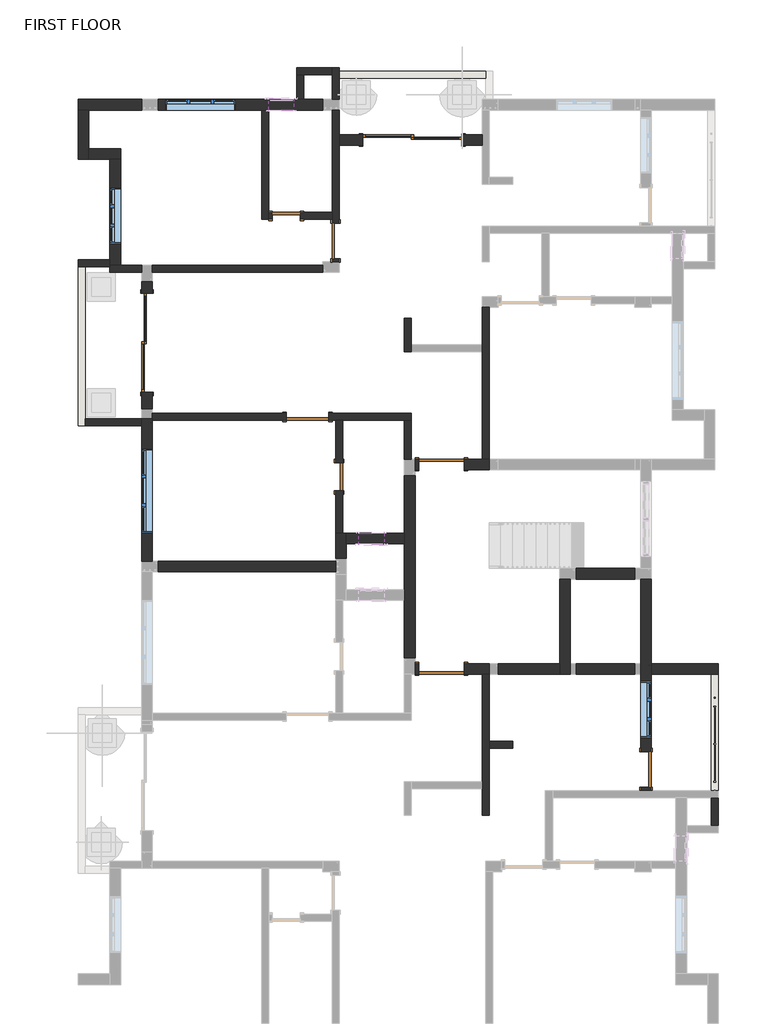
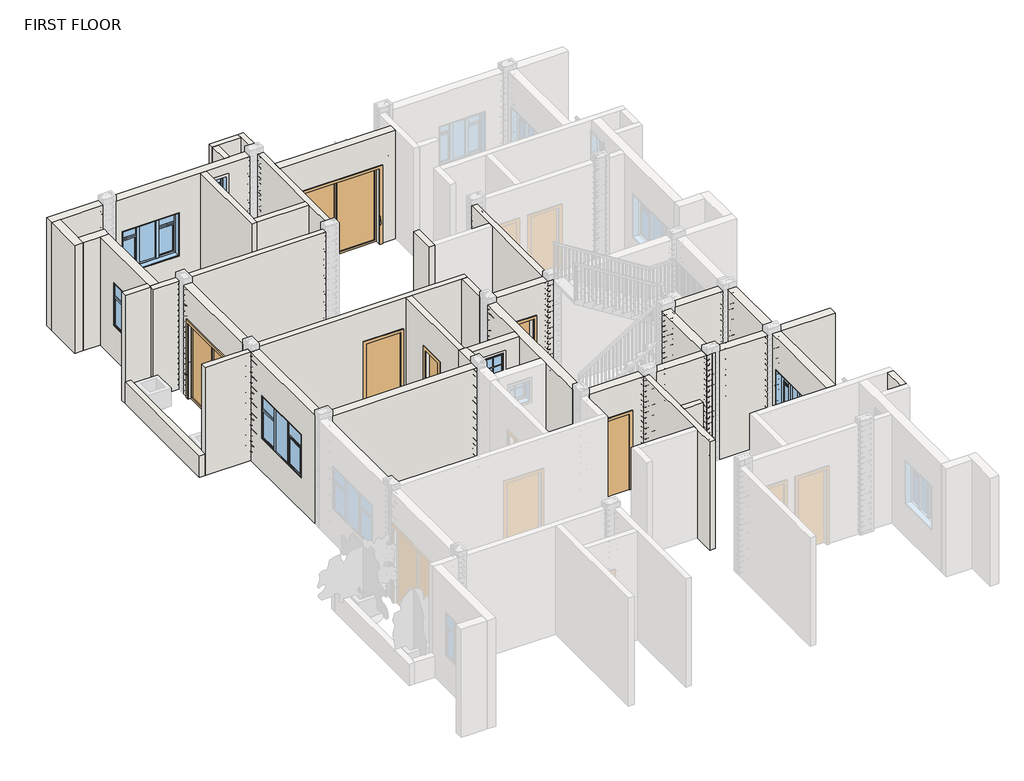
# One storey, part 2 of 10: 41 walls, 9 doors, 6 windows.
"""IFC4 building model written with IfcOpenShell, lengths in millimetres."""

from ifc_helpers import new_model, si_unit, frame, origin, place, context, project, spatial, polyline, outline, extrude, faceted_brep, transform, mapped, element, save
from components import door_double_sliding_7_x7_ddbaaa7c, door_e2b13fe9, door_bb98abfd, single_flush_2_x7_5ca4d175, door_ddcbdd8b, door_49933fe7, single_flush_3_x7_686f89d2, window_casement_triple_side_transom_4_x4_2_fd24aed3, window_casement_triple_side_transom_5_x4_f59ddf0b, window_casement_triple_side_transom_6_x4_596ba82f, window_6ec6991e

model = new_model("IFC4")

# Units and contexts
model_context = context("Model", 3, world=origin())
ifc_project = project(units=[si_unit("LENGTHUNIT", "METRE", prefix="MILLI")], contexts=[model_context])

# Site, building, storey
site = spatial("IfcSite", under=ifc_project)
building = spatial("IfcBuilding", under=site)
storey = spatial("IfcBuildingStorey", under=building, Name="FIRST FLOOR", Elevation=3200.4)

# Doors
placement = place(None, origin())
door_double_sliding_7_x7_shape = door_double_sliding_7_x7_ddbaaa7c(model_context)
element("IfcDoor", 1, ObjectType="Door-Double-Sliding : 7'X7'", at=placement, inside=storey, context=model_context, shape_type="MappedRepresentation", body=[
    mapped(door_double_sliding_7_x7_shape, transform((-403.8333787, 9140.759934, 3200.4), x_axis=(1.0, 0.0, 0.0), y_axis=(0.0, 1.0, 0.0), z_axis=(0.0, 0.0, 1.0))),
])
element("IfcDoor", 2, ObjectType="Door-Double-Sliding : 7'X7'", at=placement, inside=storey, context=model_context, shape_type="MappedRepresentation", body=[
    mapped(door_double_sliding_7_x7_shape, transform((-6010.8833787, 4886.259934, 3200.4), x_axis=(0.0, 1.0, 0.0), y_axis=(-1.0, 0.0, 0.0), z_axis=(0.0, 0.0, 1.0))),
])
door_shape = door_e2b13fe9(model_context)
element("IfcDoor", 3, ObjectType="Single-Flush : 2'6\"X7'", at=placement, inside=storey, context=model_context, shape_type="MappedRepresentation", body=[
    mapped(door_shape, transform((-2061.1833787, 7083.359934, 3200.4), x_axis=(0.0, -1.0, 0.0), y_axis=(1.0, 0.0, 0.0), z_axis=(0.0, 0.0, 1.0))),
])
door_2_shape = door_bb98abfd(model_context)
element("IfcDoor", 4, ObjectType="Single-Flush : 2'6\"X7'", at=placement, inside=storey, context=model_context, shape_type="MappedRepresentation", body=[
    mapped(door_2_shape, transform((4644.4166213, -4333.940066, 3200.4), x_axis=(0.0, -1.0, 0.0), y_axis=(1.0, 0.0, 0.0), z_axis=(0.0, 0.0, 1.0))),
])
single_flush_2_x7_shape = single_flush_2_x7_5ca4d175(model_context)
element("IfcDoor", 5, ObjectType="Single-Flush : 2'X7'", at=placement, inside=storey, context=model_context, shape_type="MappedRepresentation", body=[
    mapped(single_flush_2_x7_shape, transform((-3127.9833787, 7629.459934, 3200.4), x_axis=(-1.0, 0.0, 0.0), y_axis=(0.0, -1.0, 0.0), z_axis=(0.0, 0.0, 1.0))),
])
element("IfcDoor", 6, ObjectType="Single-Flush : 2'X7'", at=placement, inside=storey, context=model_context, shape_type="MappedRepresentation", body=[
    mapped(single_flush_2_x7_shape, transform((-1984.9833787, 1990.659934, 3200.4), x_axis=(0.0, 1.0, 0.0), y_axis=(-1.0, 0.0, 0.0), z_axis=(0.0, 0.0, 1.0))),
])
door_3_shape = door_ddcbdd8b(model_context)
element("IfcDoor", 7, ObjectType="Single-Flush : 3'3\"X7'", at=placement, inside=storey, context=model_context, shape_type="MappedRepresentation", body=[
    mapped(door_3_shape, transform((224.8166213, -2162.240066, 3200.4), x_axis=(-1.0, 0.0, 0.0), y_axis=(0.0, -1.0, 0.0), z_axis=(0.0, 0.0, 1.0))),
])
door_4_shape = door_49933fe7(model_context)
element("IfcDoor", 8, ObjectType="Single-Flush : 3'3\"X7'", at=placement, inside=storey, context=model_context, shape_type="MappedRepresentation", body=[
    mapped(door_4_shape, transform((224.8166213, 2257.359934, 3200.4), x_axis=(-1.0, 0.0, 0.0), y_axis=(0.0, -1.0, 0.0), z_axis=(0.0, 0.0, 1.0))),
])
single_flush_3_x7_shape = single_flush_3_x7_686f89d2(model_context)
element("IfcDoor", 9, ObjectType="Single-Flush : 3'X7'", at=placement, inside=storey, context=model_context, shape_type="MappedRepresentation", body=[
    mapped(single_flush_3_x7_shape, transform((-2670.7833787, 3286.059934, 3200.4), x_axis=(1.0, 0.0, 0.0), y_axis=(0.0, 1.0, 0.0), z_axis=(0.0, 0.0, 1.0))),
])

# Walls
element("IfcWall", 10, ObjectType="6\"", at=placement, inside=storey, context=model_context, shape_type="Brep", body=[
    faceted_brep([(-3661.3833787, 9915.459934, 3200.4), (-3661.3833787, 7553.259934, 3200.4), (-3661.3833787, 7553.259934, 6248.4), (-3661.3833787, 9915.459934, 6248.4), (-3508.9833787, 9915.459934, 3200.4), (-3508.9833787, 9915.459934, 5334.0), (-3508.9833787, 9915.459934, 5943.6), (-3508.9833787, 9915.459934, 6248.4), (-3508.9833787, 7705.659934, 6248.4), (-3508.9833787, 7553.259934, 6248.4), (-3508.9833787, 7553.259934, 3200.4), (-3508.9833787, 7705.659934, 3200.4)], [[[0, 1, 2, 3]], [[4, 5, 6, 7, 8, 9, 10, 11]], [[1, 0, 4, 11, 10]], [[3, 2, 9, 8, 7]], [[0, 3, 7, 6, 5, 4]], [[2, 1, 10, 9]]]),
])
element("IfcWall", 11, ObjectType="6\"", at=placement, inside=storey, context=model_context, shape_type="SweptSolid", body=[
    extrude(outline(polyline([(3200.4, -3508.9833787), (3200.4, -3432.7833787), (5334.0, -3432.7833787), (5334.0, -2823.1833787), (3200.4, -2823.1833787), (3200.4, -2137.3833787), (6248.4, -2137.3833787), (6248.4, -3508.9833787), (3200.4, -3508.9833787)])), frame((0.0, 7553.259934, 0.0), z_axis=(0.0, 1.0, 0.0), x_axis=(0.0, 0.0, 1.0)), (0.0, 0.0, 1.0), 152.4),
])
element("IfcWall", 12, ObjectType="6\"", at=placement, inside=storey, context=model_context, shape_type="Brep", body=[
    faceted_brep([(-2137.3833787, 6702.359934, 5334.0), (-2137.3833787, 6702.359934, 3200.4), (-2137.3833787, 6638.859934, 3200.4), (-2137.3833787, 6638.859934, 6248.4), (-2137.3833787, 7553.259934, 6248.4), (-2137.3833787, 7705.659934, 6248.4), (-2137.3833787, 9915.459934, 6248.4), (-2137.3833787, 9915.459934, 3200.4), (-2137.3833787, 7705.659934, 3200.4), (-2137.3833787, 7553.259934, 3200.4), (-2137.3833787, 7464.359934, 3200.4), (-2137.3833787, 7464.359934, 5334.0), (-1984.9833787, 6638.859934, 3200.4), (-1984.9833787, 6702.359934, 3200.4), (-1984.9833787, 6702.359934, 5334.0), (-1984.9833787, 7464.359934, 5334.0), (-1984.9833787, 7464.359934, 3200.4), (-1984.9833787, 9153.459934, 3200.4), (-1984.9833787, 9382.059934, 3200.4), (-1984.9833787, 9915.459934, 3200.4), (-1984.9833787, 9915.459934, 6248.4), (-1984.9833787, 9382.059934, 6248.4), (-1984.9833787, 9153.459934, 6248.4), (-1984.9833787, 6638.859934, 6248.4)], [[[0, 1, 2, 3, 4, 5, 6, 7, 8, 9, 10, 11]], [[12, 13, 14, 15, 16, 17, 18, 19, 20, 21, 22, 23]], [[2, 1, 13, 12]], [[10, 9, 8, 7, 19, 18, 17, 16]], [[3, 2, 12, 23]], [[6, 5, 4, 3, 23, 22, 21, 20]], [[7, 6, 20, 19]], [[14, 13, 1, 0]], [[15, 14, 0, 11]], [[16, 15, 11, 10]]]),
])
element("IfcWall", 13, ObjectType="6\"", at=placement, inside=storey, context=model_context, shape_type="Brep", body=[
    faceted_brep([(1101.1166213, 5648.259934, 3200.4), (1101.1166213, 4848.159934, 3200.4), (1101.1166213, 4695.759934, 3200.4), (1101.1166213, 2371.659934, 3200.4), (1101.1166213, 2371.659934, 6248.4), (1101.1166213, 4695.759934, 6248.4), (1101.1166213, 4848.159934, 6248.4), (1101.1166213, 5648.259934, 6248.4), (1253.5166213, 5648.259934, 3200.4), (1253.5166213, 5648.259934, 6248.4), (1253.5166213, 2371.659934, 6248.4), (1253.5166213, 2371.659934, 3200.4)], [[[0, 1, 2, 3, 4, 5, 6, 7]], [[8, 9, 10, 11]], [[3, 2, 1, 0, 8, 11]], [[7, 6, 5, 4, 10, 9]], [[0, 7, 9, 8]], [[4, 3, 11, 10]]]),
])
element("IfcWall", 14, ObjectType="6\"", at=placement, inside=storey, context=model_context, shape_type="Brep", body=[
    faceted_brep([(-575.2833787, 5419.659934, 3200.4), (-575.2833787, 4695.759934, 3200.4), (-575.2833787, 4695.759934, 6248.4), (-575.2833787, 5419.659934, 6248.4), (-422.8833787, 5419.659934, 3200.4), (-422.8833787, 5419.659934, 6248.4), (-422.8833787, 4848.159934, 6248.4), (-422.8833787, 4695.759934, 6248.4), (-422.8833787, 4695.759934, 3200.4), (-422.8833787, 4848.159934, 3200.4)], [[[0, 1, 2, 3]], [[4, 5, 6, 7, 8, 9]], [[1, 0, 4, 9, 8]], [[3, 2, 7, 6, 5]], [[0, 3, 5, 4]], [[2, 1, 8, 7]]]),
])
element("IfcWall", 15, ObjectType="6\"", at=placement, inside=storey, context=model_context, shape_type="Brep", body=[
    faceted_brep([(-2213.5833787, 3209.859934, 5334.0), (-2213.5833787, 3209.859934, 3200.4), (-2061.1833787, 3209.859934, 3200.4), (-1908.7833787, 3209.859934, 3200.4), (-575.2833787, 3209.859934, 3200.4), (-422.8833787, 3209.859934, 3200.4), (-422.8833787, 3209.859934, 6248.4), (-575.2833787, 3209.859934, 6248.4), (-1908.7833787, 3209.859934, 6248.4), (-2061.1833787, 3209.859934, 6248.4), (-6023.5833787, 3209.859934, 6248.4), (-6023.5833787, 3209.859934, 3200.4), (-3127.9833787, 3209.859934, 3200.4), (-3127.9833787, 3209.859934, 5334.0), (-422.8833787, 3362.259934, 3200.4), (-2213.5833787, 3362.259934, 3200.4), (-2213.5833787, 3362.259934, 5334.0), (-3127.9833787, 3362.259934, 5334.0), (-3127.9833787, 3362.259934, 3200.4), (-6023.5833787, 3362.259934, 3200.4), (-6023.5833787, 3362.259934, 6248.4), (-422.8833787, 3362.259934, 6248.4), (-6023.5833787, 3247.959934, 3200.4), (-6023.5833787, 3247.959934, 6248.4)], [[[0, 1, 2, 3, 4, 5, 6, 7, 8, 9, 10, 11, 12, 13]], [[14, 15, 16, 17, 18, 19, 20, 21]], [[12, 11, 22, 19, 18]], [[5, 4, 3, 2, 1, 15, 14]], [[10, 9, 8, 7, 6, 21, 20, 23]], [[6, 5, 14, 21]], [[16, 15, 1, 0]], [[17, 16, 0, 13]], [[18, 17, 13, 12]], [[11, 10, 23, 20, 19, 22]]]),
])
element("IfcWall", 16, ObjectType="6\"", at=placement, inside=storey, context=model_context, shape_type="SweptSolid", body=[
    extrude(outline(polyline([(-6023.5833787, 6562.659934), (-2340.5833787, 6562.659934), (-2340.5833787, 6410.259934), (-6023.5833787, 6410.259934), (-6023.5833787, 6562.659934)])), frame((0.0, 0.0, 3200.4), z_axis=(0.0, 0.0, 1.0), x_axis=(1.0, 0.0, 0.0)), (0.0, 0.0, 1.0), 3048.0),
])
element("IfcWall", 17, ObjectType="6\"", at=placement, inside=storey, context=model_context, shape_type="Brep", body=[
    faceted_brep([(-6252.1833787, 6562.659934, 3200.4), (-6709.3833787, 6562.659934, 3200.4), (-6937.9833787, 6562.659934, 3200.4), (-6937.9833787, 6562.659934, 6248.4), (-6709.3833787, 6562.659934, 6248.4), (-6252.1833787, 6562.659934, 6248.4), (-6252.1833787, 6410.259934, 3200.4), (-6252.1833787, 6410.259934, 6248.4), (-6937.9833787, 6410.259934, 6248.4), (-6937.9833787, 6410.259934, 3200.4), (-6937.9833787, 6524.559934, 3200.4), (-6937.9833787, 6524.559934, 6248.4)], [[[0, 1, 2, 3, 4, 5]], [[6, 7, 8, 9]], [[2, 1, 0, 6, 9, 10]], [[5, 4, 3, 11, 8, 7]], [[0, 5, 7, 6]], [[3, 2, 10, 9, 8, 11]]]),
])
element("IfcWall", 18, ObjectType="6\"", at=placement, inside=storey, context=model_context, shape_type="SweptSolid", body=[
    extrude(outline(polyline([(3209.859934, 3200.4), (2295.459934, 3200.4), (2295.459934, 5334.0), (1685.859934, 5334.0), (1685.859934, 3200.4), (771.459934, 3200.4), (771.459934, 6248.4), (3209.859934, 6248.4), (3209.859934, 3200.4)])), frame((-2061.1833787, 0.0, 0.0), z_axis=(1.0, 0.0, 0.0), x_axis=(0.0, 1.0, 0.0)), (0.0, 0.0, 1.0), 152.4),
])
element("IfcWall", 19, ObjectType="6\"", at=placement, inside=storey, context=model_context, shape_type="SweptSolid", body=[
    extrude(outline(polyline([(-575.2833787, 2371.659934), (-575.2833787, 3209.859934), (-422.8833787, 3209.859934), (-422.8833787, 2371.659934), (-575.2833787, 2371.659934)])), frame((0.0, 0.0, 3200.4), z_axis=(0.0, 0.0, 1.0), x_axis=(1.0, 0.0, 0.0)), (0.0, 0.0, 1.0), 3048.0),
])
element("IfcWall", 20, ObjectType="6\"", at=placement, inside=storey, context=model_context, shape_type="Brep", body=[
    faceted_brep([(1101.1166213, -2276.540066, 3200.4), (1101.1166213, -4600.640066, 3200.4), (1101.1166213, -4753.040066, 3200.4), (1101.1166213, -5324.540066, 3200.4), (1101.1166213, -5324.540066, 6248.4), (1101.1166213, -4753.040066, 6248.4), (1101.1166213, -4600.640066, 6248.4), (1101.1166213, -2276.540066, 6248.4), (1253.5166213, -2276.540066, 3200.4), (1253.5166213, -2276.540066, 6248.4), (1253.5166213, -3724.340066, 6248.4), (1253.5166213, -3876.740066, 6248.4), (1253.5166213, -5324.540066, 6248.4), (1253.5166213, -5324.540066, 3200.4), (1253.5166213, -3876.740066, 3200.4), (1253.5166213, -3724.340066, 3200.4)], [[[0, 1, 2, 3, 4, 5, 6, 7]], [[8, 9, 10, 11, 12, 13, 14, 15]], [[3, 2, 1, 0, 8, 15, 14, 13]], [[4, 3, 13, 12]], [[7, 6, 5, 4, 12, 11, 10, 9]], [[0, 7, 9, 8]]]),
])
element("IfcWall", 21, ObjectType="6\"", at=placement, inside=storey, context=model_context, shape_type="SweptSolid", body=[
    extrude(outline(polyline([(1761.5166213, -3876.740066), (1253.5166213, -3876.740066), (1253.5166213, -3724.340066), (1761.5166213, -3724.340066), (1761.5166213, -3876.740066)])), frame((0.0, 0.0, 3200.4), z_axis=(0.0, 0.0, 1.0), x_axis=(1.0, 0.0, 0.0)), (0.0, 0.0, 1.0), 3048.0),
])
element("IfcWall", 22, ObjectType="6\"", at=placement, inside=storey, context=model_context, shape_type="Brep", body=[
    faceted_brep([(6054.1166213, -2276.540066, 3200.4), (6054.1166213, -4791.140066, 3200.4), (6054.1166213, -4943.540066, 3200.4), (6054.1166213, -4943.540066, 3810.0), (6054.1166213, -4791.140066, 3810.0), (6054.1166213, -2276.540066, 3810.0), (6206.5166213, -2276.540066, 3200.4), (6206.5166213, -2276.540066, 3810.0), (6206.5166213, -4791.140066, 3810.0), (6206.5166213, -4943.540066, 3810.0), (6206.5166213, -4943.540066, 3200.4)], [[[0, 1, 2, 3, 4, 5]], [[6, 7, 8, 9, 10]], [[2, 1, 0, 6, 10]], [[5, 4, 3, 9, 8, 7]], [[0, 5, 7, 6]], [[3, 2, 10, 9]]]),
])
element("IfcWall", 23, ObjectType="6\"", at=placement, inside=storey, context=model_context, shape_type="SweptSolid", body=[
    extrude(outline(polyline([(-1984.9833787, 10753.659934), (1177.3166213, 10753.659934), (1177.3166213, 10601.259934), (-1984.9833787, 10601.259934), (-1984.9833787, 10753.659934)])), frame((0.0, 0.0, 3200.4), z_axis=(0.0, 0.0, 1.0), x_axis=(1.0, 0.0, 0.0)), (0.0, 0.0, 1.0), 609.6),
])
element("IfcWall", 24, ObjectType="6\"", at=placement, inside=storey, context=model_context, shape_type="Brep", body=[
    faceted_brep([(-1984.9833787, 10144.059934, 3200.4), (-1984.9833787, 10601.259934, 3200.4), (-1984.9833787, 10753.659934, 3200.4), (-1984.9833787, 10829.859934, 3200.4), (-1984.9833787, 10829.859934, 6248.4), (-1984.9833787, 10144.059934, 6248.4), (-2137.3833787, 10144.059934, 3200.4), (-2137.3833787, 10144.059934, 6248.4), (-2137.3833787, 10677.459934, 6248.4), (-2137.3833787, 10829.859934, 6248.4), (-2137.3833787, 10829.859934, 3200.4), (-2137.3833787, 10677.459934, 3200.4)], [[[0, 1, 2, 3, 4, 5]], [[6, 7, 8, 9, 10, 11]], [[3, 2, 1, 0, 6, 11, 10]], [[5, 4, 9, 8, 7]], [[0, 5, 7, 6]], [[4, 3, 10, 9]]]),
])
element("IfcWall", 25, ObjectType="6\"", at=placement, inside=storey, context=model_context, shape_type="Brep", body=[
    faceted_brep([(-2137.3833787, 10829.859934, 6248.4), (-2137.3833787, 10829.859934, 3200.4), (-2898.7100526, 10829.859934, 3200.4), (-2898.7100526, 10829.859934, 6248.4), (-2137.3833787, 10677.459934, 3200.4), (-2137.3833787, 10677.459934, 6248.4), (-2746.3100526, 10677.459934, 6248.4), (-2898.7100526, 10677.459934, 6248.4), (-2898.7100526, 10677.459934, 3200.4), (-2746.3100526, 10677.459934, 3200.4)], [[[0, 1, 2, 3]], [[4, 5, 6, 7, 8, 9]], [[2, 1, 4, 9, 8]], [[0, 3, 7, 6, 5]], [[3, 2, 8, 7]], [[0, 5, 4, 1]]]),
])
element("IfcWall", 26, ObjectType="6\"", at=placement, inside=storey, context=model_context, shape_type="SweptSolid", body=[
    extrude(outline(polyline([(-2898.7100526, 10144.059934), (-2898.7100526, 10677.459934), (-2746.3100526, 10677.459934), (-2746.3100526, 10144.059934), (-2898.7100526, 10144.059934)])), frame((0.0, 0.0, 3200.4), z_axis=(0.0, 0.0, 1.0), x_axis=(1.0, 0.0, 0.0)), (0.0, 0.0, 1.0), 3048.0),
])
element("IfcWall", 27, ObjectType="6\"", at=placement, inside=storey, context=model_context, shape_type="Brep", body=[
    faceted_brep([(-6937.9833787, 6676.959934, 3200.4), (-7623.7833787, 6676.959934, 3200.4), (-7623.7833787, 6676.959934, 6248.4), (-6937.9833787, 6676.959934, 6248.4), (-6937.9833787, 6524.559934, 3200.4), (-6937.9833787, 6524.559934, 6248.4), (-7623.7833787, 6524.559934, 6248.4), (-7623.7833787, 6524.559934, 3810.0), (-7623.7833787, 6524.559934, 3200.4), (-7471.3833787, 6524.559934, 3200.4), (-6937.9833787, 6562.659934, 3200.4), (-6937.9833787, 6562.659934, 6248.4)], [[[0, 1, 2, 3]], [[4, 5, 6, 7, 8, 9]], [[1, 0, 10, 4, 9, 8]], [[3, 2, 6, 5, 11]], [[0, 3, 11, 5, 4, 10]], [[2, 1, 8, 7, 6]]]),
])
element("IfcWall", 28, ObjectType="6\"", at=placement, inside=storey, context=model_context, shape_type="Brep", body=[
    faceted_brep([(-7623.7833787, 6524.559934, 3200.4), (-7623.7833787, 3095.559934, 3200.4), (-7623.7833787, 3095.559934, 3810.0), (-7623.7833787, 6524.559934, 3810.0), (-7471.3833787, 6524.559934, 3200.4), (-7471.3833787, 6524.559934, 3810.0), (-7471.3833787, 3095.559934, 3810.0), (-7471.3833787, 3095.559934, 3200.4), (-7471.3833787, 3247.959934, 3200.4)], [[[0, 1, 2, 3]], [[4, 5, 6, 7, 8]], [[1, 0, 4, 8, 7]], [[3, 2, 6, 5]], [[0, 3, 5, 4]], [[2, 1, 7, 6]]]),
])
element("IfcWall", 29, ObjectType="6\"", at=placement, inside=storey, context=model_context, shape_type="Brep", body=[
    faceted_brep([(-7471.3833787, 3095.559934, 3200.4), (-6252.1833787, 3095.559934, 3200.4), (-6252.1833787, 3095.559934, 6248.4), (-7471.3833787, 3095.559934, 6248.4), (-7471.3833787, 3095.559934, 3810.0), (-7471.3833787, 3247.959934, 3200.4), (-7471.3833787, 3247.959934, 6248.4), (-6252.1833787, 3247.959934, 6248.4), (-6252.1833787, 3247.959934, 3200.4)], [[[0, 1, 2, 3, 4]], [[5, 6, 7, 8]], [[1, 0, 5, 8]], [[3, 2, 7, 6]], [[2, 1, 8, 7]], [[0, 4, 3, 6, 5]]]),
])
element("IfcWall", 30, ObjectType="6\"", at=placement, inside=storey, context=model_context, shape_type="Brep", body=[
    faceted_brep([(6054.1166213, -4943.540066, 3200.4), (6054.1166213, -5552.4667399, 3200.4), (6054.1166213, -5552.4667399, 6248.4), (6054.1166213, -4943.540066, 6248.4), (6054.1166213, -4943.540066, 3810.0), (6206.5166213, -4943.540066, 3200.4), (6206.5166213, -4943.540066, 3810.0), (6206.5166213, -4943.540066, 6248.4), (6206.5166213, -5552.4667399, 6248.4), (6206.5166213, -5552.4667399, 3200.4)], [[[0, 1, 2, 3, 4]], [[5, 6, 7, 8, 9]], [[1, 0, 5, 9]], [[3, 2, 8, 7]], [[0, 4, 3, 7, 6, 5]], [[2, 1, 9, 8]]]),
])
element("IfcWall", 31, ObjectType="9\"", at=placement, inside=storey, context=model_context, shape_type="Brep", body=[
    faceted_brep([(-6252.1833787, 10144.059934, 3200.4), (-7623.7833787, 10144.059934, 3200.4), (-7623.7833787, 10144.059934, 6248.4), (-6252.1833787, 10144.059934, 6248.4), (-6252.1833787, 9915.459934, 3200.4), (-6252.1833787, 9915.459934, 6248.4), (-7395.1833787, 9915.459934, 6248.4), (-7623.7833787, 9915.459934, 6248.4), (-7623.7833787, 9915.459934, 3200.4), (-7395.1833787, 9915.459934, 3200.4)], [[[0, 1, 2, 3]], [[4, 5, 6, 7, 8, 9]], [[1, 0, 4, 9, 8]], [[3, 2, 7, 6, 5]], [[0, 3, 5, 4]], [[2, 1, 8, 7]]]),
])
element("IfcWall", 32, ObjectType="9\"", at=placement, inside=storey, context=model_context, shape_type="Brep", body=[
    faceted_brep([(-7623.7833787, 9915.459934, 3200.4), (-7623.7833787, 8848.659934, 3200.4), (-7623.7833787, 8848.659934, 6248.4), (-7623.7833787, 9915.459934, 6248.4), (-7395.1833787, 9915.459934, 3200.4), (-7395.1833787, 9915.459934, 6248.4), (-7395.1833787, 9077.259934, 6248.4), (-7395.1833787, 8848.659934, 6248.4), (-7395.1833787, 8848.659934, 3200.4), (-7395.1833787, 9077.259934, 3200.4)], [[[0, 1, 2, 3]], [[4, 5, 6, 7, 8, 9]], [[1, 0, 4, 9, 8]], [[3, 2, 7, 6, 5]], [[0, 3, 5, 4]], [[2, 1, 8, 7]]]),
])
element("IfcWall", 33, ObjectType="9\"", at=placement, inside=storey, context=model_context, shape_type="Brep", body=[
    faceted_brep([(-7395.1833787, 8848.659934, 3200.4), (-6937.9833787, 8848.659934, 3200.4), (-6709.3833787, 8848.659934, 3200.4), (-6709.3833787, 8848.659934, 6248.4), (-6937.9833787, 8848.659934, 6248.4), (-7395.1833787, 8848.659934, 6248.4), (-7395.1833787, 9077.259934, 3200.4), (-7395.1833787, 9077.259934, 6248.4), (-6709.3833787, 9077.259934, 6248.4), (-6709.3833787, 9077.259934, 3200.4)], [[[0, 1, 2, 3, 4, 5]], [[6, 7, 8, 9]], [[2, 1, 0, 6, 9]], [[5, 4, 3, 8, 7]], [[0, 5, 7, 6]], [[3, 2, 9, 8]]]),
])
element("IfcWall", 34, ObjectType="9\"", at=placement, inside=storey, context=model_context, shape_type="Brep", body=[
    faceted_brep([(-6937.9833787, 8848.659934, 3200.4), (-6937.9833787, 6676.959934, 3200.4), (-6937.9833787, 6562.659934, 3200.4), (-6937.9833787, 6562.659934, 6248.4), (-6937.9833787, 6676.959934, 6248.4), (-6937.9833787, 8848.659934, 6248.4), (-6937.9833787, 8239.059934, 5334.0), (-6937.9833787, 7019.859934, 5334.0), (-6937.9833787, 7019.859934, 4114.8), (-6937.9833787, 8239.059934, 4114.8), (-6709.3833787, 8848.659934, 3200.4), (-6709.3833787, 8848.659934, 6248.4), (-6709.3833787, 6562.659934, 6248.4), (-6709.3833787, 6562.659934, 3200.4), (-6709.3833787, 8239.059934, 5334.0), (-6709.3833787, 8239.059934, 4114.8), (-6709.3833787, 7019.859934, 4114.8), (-6709.3833787, 7019.859934, 5334.0)], [[[0, 1, 2, 3, 4, 5], [6, 7, 8, 9]], [[10, 11, 12, 13], [14, 15, 16, 17]], [[2, 1, 0, 10, 13]], [[5, 4, 3, 12, 11]], [[0, 5, 11, 10]], [[3, 2, 13, 12]], [[15, 14, 6, 9]], [[16, 15, 9, 8]], [[17, 16, 8, 7]], [[14, 17, 7, 6]]]),
])
element("IfcWall", 35, ObjectType="9\"", at=placement, inside=storey, context=model_context, shape_type="SweptSolid", body=[
    extrude(outline(polyline([(6207.059934, 3200.4), (5953.059934, 3200.4), (5953.059934, 5334.0), (3819.459934, 5334.0), (3819.459934, 3200.4), (3463.859934, 3200.4), (3463.859934, 6248.4), (6207.059934, 6248.4), (6207.059934, 3200.4)])), frame((-6252.1833787, 0.0, 0.0), z_axis=(1.0, 0.0, 0.0), x_axis=(0.0, 1.0, 0.0)), (0.0, 0.0, 1.0), 228.6),
])
element("IfcWall", 36, ObjectType="9\"", at=placement, inside=storey, context=model_context, shape_type="Brep", body=[
    faceted_brep([(-6252.1833787, 3247.959934, 3200.4), (-6252.1833787, 3095.559934, 3200.4), (-6252.1833787, 161.859934, 3200.4), (-6252.1833787, 161.859934, 6248.4), (-6252.1833787, 3095.559934, 6248.4), (-6252.1833787, 3247.959934, 6248.4), (-6252.1833787, 2600.259934, 5334.0), (-6252.1833787, 771.459934, 5334.0), (-6252.1833787, 771.459934, 4114.8), (-6252.1833787, 2600.259934, 4114.8), (-6023.5833787, 3247.959934, 3200.4), (-6023.5833787, 3247.959934, 6248.4), (-6023.5833787, 3209.859934, 6248.4), (-6023.5833787, 161.859934, 6248.4), (-6023.5833787, 161.859934, 3200.4), (-6023.5833787, 3209.859934, 3200.4), (-6023.5833787, 2600.259934, 5334.0), (-6023.5833787, 2600.259934, 4114.8), (-6023.5833787, 771.459934, 4114.8), (-6023.5833787, 771.459934, 5334.0)], [[[0, 1, 2, 3, 4, 5], [6, 7, 8, 9]], [[10, 11, 12, 13, 14, 15], [16, 17, 18, 19]], [[2, 1, 0, 10, 15, 14]], [[3, 2, 14, 13]], [[5, 4, 3, 13, 12, 11]], [[0, 5, 11, 10]], [[17, 16, 6, 9]], [[18, 17, 9, 8]], [[19, 18, 8, 7]], [[16, 19, 7, 6]]]),
])
element("IfcWall", 37, ObjectType="9\"", at=placement, inside=storey, context=model_context, shape_type="Brep", body=[
    faceted_brep([(4758.7166213, -4791.140066, 3200.4), (4758.7166213, -4714.940066, 3200.4), (4758.7166213, -4714.940066, 5334.0), (4758.7166213, -3952.940066, 5334.0), (4758.7166213, -3952.940066, 3200.4), (4758.7166213, -2276.540066, 3200.4), (4758.7166213, -2047.940066, 3200.4), (4758.7166213, -219.140066, 3200.4), (4758.7166213, -219.140066, 6248.4), (4758.7166213, -2047.940066, 6248.4), (4758.7166213, -2276.540066, 6248.4), (4758.7166213, -4791.140066, 6248.4), (4758.7166213, -3648.140066, 5334.0), (4758.7166213, -2428.940066, 5334.0), (4758.7166213, -2428.940066, 4114.8), (4758.7166213, -3648.140066, 4114.8), (4530.1166213, -4714.940066, 5334.0), (4530.1166213, -4714.940066, 3200.4), (4530.1166213, -4791.140066, 3200.4), (4530.1166213, -4791.140066, 6248.4), (4530.1166213, -219.140066, 6248.4), (4530.1166213, -219.140066, 3200.4), (4530.1166213, -3952.940066, 3200.4), (4530.1166213, -3952.940066, 5334.0), (4530.1166213, -3648.140066, 5334.0), (4530.1166213, -3648.140066, 4114.8), (4530.1166213, -2428.940066, 4114.8), (4530.1166213, -2428.940066, 5334.0)], [[[0, 1, 2, 3, 4, 5, 6, 7, 8, 9, 10, 11], [12, 13, 14, 15]], [[16, 17, 18, 19, 20, 21, 22, 23], [24, 25, 26, 27]], [[22, 21, 7, 6, 5, 4]], [[18, 17, 1, 0]], [[8, 7, 21, 20]], [[11, 10, 9, 8, 20, 19]], [[0, 11, 19, 18]], [[2, 1, 17, 16]], [[3, 2, 16, 23]], [[4, 3, 23, 22]], [[25, 24, 12, 15]], [[26, 25, 15, 14]], [[27, 26, 14, 13]], [[24, 27, 13, 12]]]),
])
element("IfcWall", 38, ObjectType="9\"", at=placement, inside=storey, context=model_context, shape_type="Brep", body=[
    faceted_brep([(6206.5166213, -2047.940066, 3200.4), (4758.7166213, -2047.940066, 3200.4), (4758.7166213, -2047.940066, 6248.4), (6206.5166213, -2047.940066, 6248.4), (6206.5166213, -2276.540066, 3200.4), (6206.5166213, -2276.540066, 3810.0), (6206.5166213, -2276.540066, 6248.4), (4758.7166213, -2276.540066, 6248.4), (4758.7166213, -2276.540066, 3200.4), (6054.1166213, -2276.540066, 3200.4)], [[[0, 1, 2, 3]], [[4, 5, 6, 7, 8, 9]], [[1, 0, 4, 9, 8]], [[3, 2, 7, 6]], [[2, 1, 8, 7]], [[0, 3, 6, 5, 4]]]),
])
element("IfcWall", 39, ObjectType="9\"", at=placement, inside=storey, context=model_context, shape_type="Brep", body=[
    faceted_brep([(-346.6833787, 2143.059934, 3200.4), (-270.4833787, 2143.059934, 3200.4), (-270.4833787, 2143.059934, 5334.0), (720.1166213, 2143.059934, 5334.0), (720.1166213, 2143.059934, 3200.4), (1253.5166213, 2143.059934, 3200.4), (1253.5166213, 2143.059934, 6248.4), (-346.6833787, 2143.059934, 6248.4), (-270.4833787, 2371.659934, 5334.0), (-270.4833787, 2371.659934, 3200.4), (-346.6833787, 2371.659934, 3200.4), (-346.6833787, 2371.659934, 6248.4), (1101.1166213, 2371.659934, 6248.4), (1253.5166213, 2371.659934, 6248.4), (1253.5166213, 2371.659934, 3200.4), (1101.1166213, 2371.659934, 3200.4), (720.1166213, 2371.659934, 3200.4), (720.1166213, 2371.659934, 5334.0)], [[[0, 1, 2, 3, 4, 5, 6, 7]], [[8, 9, 10, 11, 12, 13, 14, 15, 16, 17]], [[10, 9, 1, 0]], [[16, 15, 14, 5, 4]], [[7, 6, 13, 12, 11]], [[0, 7, 11, 10]], [[6, 5, 14, 13]], [[2, 1, 9, 8]], [[3, 2, 8, 17]], [[4, 3, 17, 16]]]),
])
element("IfcWall", 40, ObjectType="9\"", at=placement, inside=storey, context=model_context, shape_type="Brep", body=[
    faceted_brep([(-2340.5833787, 10144.059934, 3200.4), (-2746.3100526, 10144.059934, 3200.4), (-2898.7100526, 10144.059934, 3200.4), (-5896.5833787, 10144.059934, 3200.4), (-5896.5833787, 10144.059934, 6248.4), (-2898.7100526, 10144.059934, 6248.4), (-2746.3100526, 10144.059934, 6248.4), (-2340.5833787, 10144.059934, 6248.4), (-4220.1833787, 10144.059934, 5334.0), (-5744.1833787, 10144.059934, 5334.0), (-5744.1833787, 10144.059934, 4114.8), (-4220.1833787, 10144.059934, 4114.8), (-2962.8833787, 10144.059934, 5943.6), (-3508.9833787, 10144.059934, 5943.6), (-3508.9833787, 10144.059934, 5334.0), (-2962.8833787, 10144.059934, 5334.0), (-2340.5833787, 9915.459934, 3200.4), (-2340.5833787, 9915.459934, 6248.4), (-3508.9833787, 9915.459934, 6248.4), (-3661.3833787, 9915.459934, 6248.4), (-5896.5833787, 9915.459934, 6248.4), (-5896.5833787, 9915.459934, 3200.4), (-3661.3833787, 9915.459934, 3200.4), (-3508.9833787, 9915.459934, 3200.4), (-4220.1833787, 9915.459934, 5334.0), (-4220.1833787, 9915.459934, 4114.8), (-5744.1833787, 9915.459934, 4114.8), (-5744.1833787, 9915.459934, 5334.0), (-2962.8833787, 9915.459934, 5943.6), (-2962.8833787, 9915.459934, 5334.0), (-3508.9833787, 9915.459934, 5334.0), (-3508.9833787, 9915.459934, 5943.6)], [[[0, 1, 2, 3, 4, 5, 6, 7], [8, 9, 10, 11], [12, 13, 14, 15]], [[16, 17, 18, 19, 20, 21, 22, 23], [24, 25, 26, 27], [28, 29, 30, 31]], [[3, 2, 1, 0, 16, 23, 22, 21]], [[4, 3, 21, 20]], [[7, 6, 5, 4, 20, 19, 18, 17]], [[0, 7, 17, 16]], [[25, 24, 8, 11]], [[26, 25, 11, 10]], [[27, 26, 10, 9]], [[24, 27, 9, 8]], [[29, 28, 12, 15]], [[30, 29, 15, 14]], [[31, 30, 14, 13]], [[28, 31, 13, 12]]]),
])
element("IfcWall", 41, ObjectType="9\"", at=placement, inside=storey, context=model_context, shape_type="SweptSolid", body=[
    extrude(outline(polyline([(5334.0, 662.9666213), (3200.4, 662.9666213), (3200.4, 1101.1166213), (6248.4, 1101.1166213), (6248.4, -1984.9833787), (3200.4, -1984.9833787), (3200.4, -1470.6333787), (5334.0, -1470.6333787), (5334.0, 662.9666213)])), frame((0.0, 9153.459934, 0.0), z_axis=(0.0, 1.0, 0.0), x_axis=(0.0, 0.0, 1.0)), (0.0, 0.0, 1.0), 228.6),
])
element("IfcWall", 42, ObjectType="9\"", at=placement, inside=storey, context=model_context, shape_type="Brep", body=[
    faceted_brep([(-575.2833787, 2016.059934, 3200.4), (-575.2833787, 771.459934, 3200.4), (-575.2833787, 542.859934, 3200.4), (-575.2833787, -447.740066, 3200.4), (-575.2833787, -676.340066, 3200.4), (-575.2833787, -1920.940066, 3200.4), (-575.2833787, -1920.940066, 6248.4), (-575.2833787, -676.340066, 6248.4), (-575.2833787, -447.740066, 6248.4), (-575.2833787, 542.859934, 6248.4), (-575.2833787, 771.459934, 6248.4), (-575.2833787, 2016.059934, 6248.4), (-346.6833787, 2016.059934, 3200.4), (-346.6833787, 2016.059934, 6248.4), (-346.6833787, -1920.940066, 6248.4), (-346.6833787, -1920.940066, 3200.4)], [[[0, 1, 2, 3, 4, 5, 6, 7, 8, 9, 10, 11]], [[12, 13, 14, 15]], [[5, 4, 3, 2, 1, 0, 12, 15]], [[6, 5, 15, 14]], [[11, 10, 9, 8, 7, 6, 14, 13]], [[0, 11, 13, 12]]]),
])
element("IfcWall", 43, ObjectType="9\"", at=placement, inside=storey, context=model_context, shape_type="SweptSolid", body=[
    extrude(outline(polyline([(3200.4, -575.2833787), (6248.4, -575.2833787), (6248.4, -1832.5833787), (3200.4, -1832.5833787), (3200.4, -575.2833787)]), holes=[polyline([(5943.6, -1559.5333787), (5943.6, -1013.4333787), (5334.0, -1013.4333787), (5334.0, -1559.5333787), (5943.6, -1559.5333787)])]), frame((0.0, 542.859934, 0.0), z_axis=(0.0, 1.0, 0.0), x_axis=(0.0, 0.0, 1.0)), (0.0, 0.0, 1.0), 228.6),
])
element("IfcWall", 44, ObjectType="9\"", at=placement, inside=storey, context=model_context, shape_type="Brep", body=[
    faceted_brep([(-2061.1833787, 771.459934, 3200.4), (-2061.1833787, 225.359934, 3200.4), (-2061.1833787, 225.359934, 6248.4), (-2061.1833787, 771.459934, 6248.4), (-1832.5833787, 771.459934, 3200.4), (-1832.5833787, 771.459934, 6248.4), (-1832.5833787, 542.859934, 6248.4), (-1832.5833787, 225.359934, 6248.4), (-1832.5833787, 225.359934, 3200.4), (-1832.5833787, 542.859934, 3200.4), (-1908.7833787, 771.459934, 3200.4), (-1908.7833787, 771.459934, 6248.4)], [[[0, 1, 2, 3]], [[4, 5, 6, 7, 8, 9]], [[1, 0, 10, 4, 9, 8]], [[2, 1, 8, 7]], [[3, 2, 7, 6, 5, 11]], [[0, 3, 11, 5, 4, 10]]]),
])
element("IfcWall", 45, ObjectType="9\"", at=placement, inside=storey, context=model_context, shape_type="SweptSolid", body=[
    extrude(outline(polyline([(-2061.1833787, -66.740066), (-5896.5833787, -66.740066), (-5896.5833787, 161.859934), (-2061.1833787, 161.859934), (-2061.1833787, -66.740066)])), frame((0.0, 0.0, 3200.4), z_axis=(0.0, 0.0, 1.0), x_axis=(1.0, 0.0, 0.0)), (0.0, 0.0, 1.0), 3048.0),
])
element("IfcWall", 46, ObjectType="9\"", at=placement, inside=storey, context=model_context, shape_type="SweptSolid", body=[
    extrude(outline(polyline([(3133.1166213, 9.459934), (4403.1166213, 9.459934), (4403.1166213, -219.140066), (3133.1166213, -219.140066), (3133.1166213, 9.459934)])), frame((0.0, 0.0, 3200.4), z_axis=(0.0, 0.0, 1.0), x_axis=(1.0, 0.0, 0.0)), (0.0, 0.0, 1.0), 3048.0),
])
element("IfcWall", 47, ObjectType="9\"", at=placement, inside=storey, context=model_context, shape_type="Brep", body=[
    faceted_brep([(2777.5166213, -219.140066, 3200.4), (2777.5166213, -2047.940066, 3200.4), (2777.5166213, -2276.540066, 3200.4), (2777.5166213, -2276.540066, 6248.4), (2777.5166213, -2047.940066, 6248.4), (2777.5166213, -219.140066, 6248.4), (3006.1166213, -219.140066, 3200.4), (3006.1166213, -219.140066, 6248.4), (3006.1166213, -2276.540066, 6248.4), (3006.1166213, -2276.540066, 3200.4)], [[[0, 1, 2, 3, 4, 5]], [[6, 7, 8, 9]], [[2, 1, 0, 6, 9]], [[5, 4, 3, 8, 7]], [[0, 5, 7, 6]], [[3, 2, 9, 8]]]),
])
element("IfcWall", 48, ObjectType="9\"", at=placement, inside=storey, context=model_context, shape_type="SweptSolid", body=[
    extrude(outline(polyline([(3133.1166213, -2047.940066), (4403.1166213, -2047.940066), (4403.1166213, -2276.540066), (3133.1166213, -2276.540066), (3133.1166213, -2047.940066)])), frame((0.0, 0.0, 3200.4), z_axis=(0.0, 0.0, 1.0), x_axis=(1.0, 0.0, 0.0)), (0.0, 0.0, 1.0), 3048.0),
])
element("IfcWall", 49, ObjectType="9\"", at=placement, inside=storey, context=model_context, shape_type="SweptSolid", body=[
    extrude(outline(polyline([(1456.7166213, -2047.940066), (2777.5166213, -2047.940066), (2777.5166213, -2276.540066), (1456.7166213, -2276.540066), (1456.7166213, -2047.940066)])), frame((0.0, 0.0, 3200.4), z_axis=(0.0, 0.0, 1.0), x_axis=(1.0, 0.0, 0.0)), (0.0, 0.0, 1.0), 3048.0),
])
element("IfcWall", 50, ObjectType="9\"", at=placement, inside=storey, context=model_context, shape_type="Brep", body=[
    faceted_brep([(-270.4833787, -2047.940066, 5334.0), (-270.4833787, -2047.940066, 3200.4), (-346.6833787, -2047.940066, 3200.4), (-346.6833787, -2047.940066, 6248.4), (1253.5166213, -2047.940066, 6248.4), (1253.5166213, -2047.940066, 3200.4), (720.1166213, -2047.940066, 3200.4), (720.1166213, -2047.940066, 5334.0), (-346.6833787, -2276.540066, 3200.4), (-270.4833787, -2276.540066, 3200.4), (-270.4833787, -2276.540066, 5334.0), (720.1166213, -2276.540066, 5334.0), (720.1166213, -2276.540066, 3200.4), (1101.1166213, -2276.540066, 3200.4), (1253.5166213, -2276.540066, 3200.4), (1253.5166213, -2276.540066, 6248.4), (1101.1166213, -2276.540066, 6248.4), (-346.6833787, -2276.540066, 6248.4)], [[[0, 1, 2, 3, 4, 5, 6, 7]], [[8, 9, 10, 11, 12, 13, 14, 15, 16, 17]], [[6, 5, 14, 13, 12]], [[2, 1, 9, 8]], [[3, 2, 8, 17]], [[4, 3, 17, 16, 15]], [[5, 4, 15, 14]], [[10, 9, 1, 0]], [[11, 10, 0, 7]], [[12, 11, 7, 6]]]),
])

# Windows
window_casement_triple_side_transom_4_x4_2_shape = window_casement_triple_side_transom_4_x4_2_fd24aed3(model_context)
element("IfcWindow", 51, ObjectType="Window-Casement-Triple-Side-Transom : 4'X4' 2", at=placement, inside=storey, context=model_context, shape_type="MappedRepresentation", body=[
    mapped(window_casement_triple_side_transom_4_x4_2_shape, transform((-6823.6833787, 7629.459934, 3200.4), x_axis=(0.0, 1.0, 0.0), y_axis=(-1.0, 0.0, 0.0), z_axis=(0.0, 0.0, 1.0))),
])
element("IfcWindow", 52, ObjectType="Window-Casement-Triple-Side-Transom : 4'X4' 2", at=placement, inside=storey, context=model_context, shape_type="MappedRepresentation", body=[
    mapped(window_casement_triple_side_transom_4_x4_2_shape, transform((4644.4166213, -3038.540066, 3200.4), x_axis=(0.0, -1.0, 0.0), y_axis=(1.0, 0.0, 0.0), z_axis=(0.0, 0.0, 1.0))),
])
window_casement_triple_side_transom_5_x4_shape = window_casement_triple_side_transom_5_x4_f59ddf0b(model_context)
element("IfcWindow", 53, ObjectType="Window-Casement-Triple-Side-Transom : 5'X4'", at=placement, inside=storey, context=model_context, shape_type="MappedRepresentation", body=[
    mapped(window_casement_triple_side_transom_5_x4_shape, transform((-4982.1833787, 10029.759934, 3200.4), x_axis=(1.0, 0.0, 0.0), y_axis=(0.0, 1.0, 0.0), z_axis=(0.0, 0.0, 1.0))),
])
window_casement_triple_side_transom_6_x4_shape = window_casement_triple_side_transom_6_x4_596ba82f(model_context)
element("IfcWindow", 54, ObjectType="Window-Casement-Triple-Side-Transom : 6'X4'", at=placement, inside=storey, context=model_context, shape_type="MappedRepresentation", body=[
    mapped(window_casement_triple_side_transom_6_x4_shape, transform((-6137.8833787, 1685.859934, 3200.4), x_axis=(0.0, 1.0, 0.0), y_axis=(-1.0, 0.0, 0.0), z_axis=(0.0, 0.0, 1.0))),
])
window_shape = window_6ec6991e(model_context)
element("IfcWindow", 55, ObjectType="Window-Fixed : 1'9.5\"X2'", at=placement, inside=storey, context=model_context, shape_type="MappedRepresentation", body=[
    mapped(window_shape, transform((-3235.9333787, 10029.759934, 3200.4), x_axis=(1.0, 0.0, 0.0), y_axis=(0.0, 1.0, 0.0), z_axis=(0.0, 0.0, 1.0))),
])
element("IfcWindow", 56, ObjectType="Window-Fixed : 1'9.5\"X2'", at=placement, inside=storey, context=model_context, shape_type="MappedRepresentation", body=[
    mapped(window_shape, transform((-1286.4833787, 657.159934, 3200.4), x_axis=(-1.0, 0.0, 0.0), y_axis=(0.0, -1.0, 0.0), z_axis=(0.0, 0.0, 1.0))),
])

save(model, "model.ifc")

# Revit data of these elements
# Type "Door-Double-Sliding : 7'X7'"
#   Type Mark = "14"
#   Construction Type Id = "opn-d45"
#   Assembly Code = "C1020"
#   Analytic Construction = "Wood frame, double glass door "
#   Thickness = 0' - 2"
#   Thermal Resistance (R) = 1.8150 (h·ft²·°F)/BTU
#   Heat Transfer Coefficient (U) = 0.5510 BTU/(h·ft²·°F)
#   Height = 7' - 0"
#   Rail Width = 0' - 2"
#   Stiles = 0' - 2"
#   Trim Projection Ext = 0' - 1"
#   Trim Projection Int = 0' - 1"
#   Trim Width = 0' - 3"
#   Width = 7' - 0"
#   Define Thermal Properties by = 1
#   Glazing = Glass
#   Panel Material = Wood - Birch - Solid Stained Light Low Gloss
#   Trim Material = Paint - Sienna
#   Visual Light Transmittance = 0
#   Solar Heat Gain Coefficient = 0
#   Function = (empty or 0)
#   Wall Closure = (empty or 0)
# Type "Single-Flush : 2'6\"X7'"
#   Type Mark = "10"
#   Construction Type Id = "MDOOR"
#   Assembly Code = "C1020"
#   Analytic Construction = "Metal"
#   Thickness = 0' - 2"
#   Heat Transfer Coefficient (U) = 0.651978 BTU/(h·ft²·°F)
#   Height = 7' - 0"
#   Trim Projection Ext = 0' - 1"
#   Trim Projection Int = 0' - 1"
#   Trim Width = 0' - 3"
#   Width = 2' - 6"
#   Define Thermal Properties by = 1
#   Door Material = Door - Panel
#   Frame Material = Door - Frame
#   Visual Light Transmittance = 0
#   Solar Heat Gain Coefficient = 0
#   Function = (empty or 0)
#   Wall Closure = (empty or 0)
# Type "Single-Flush : 2'X7'"
#   Type Mark = "12"
#   Construction Type Id = "MDOOR"
#   Assembly Code = "C1020"
#   Analytic Construction = "Metal"
#   Thickness = 0' - 2"
#   Heat Transfer Coefficient (U) = 0.651978 BTU/(h·ft²·°F)
#   Height = 7' - 0"
#   Trim Projection Ext = 0' - 1"
#   Trim Projection Int = 0' - 1"
#   Trim Width = 0' - 3"
#   Width = 2' - 0"
#   Define Thermal Properties by = 1
#   Door Material = Door - Panel
#   Frame Material = Door - Frame
#   Visual Light Transmittance = 0
#   Solar Heat Gain Coefficient = 0
#   Function = (empty or 0)
#   Wall Closure = (empty or 0)
# Type "Single-Flush : 3'3\"X7'"
#   Type Mark = "11"
#   Construction Type Id = "MDOOR"
#   Assembly Code = "C1020"
#   Analytic Construction = "Metal"
#   Thickness = 0' - 2"
#   Heat Transfer Coefficient (U) = 0.651978 BTU/(h·ft²·°F)
#   Height = 7' - 0"
#   Trim Projection Ext = 0' - 1"
#   Trim Projection Int = 0' - 1"
#   Trim Width = 0' - 3"
#   Width = 3' - 3"
#   Define Thermal Properties by = 1
#   Door Material = Door - Panel
#   Frame Material = Door - Frame
#   Visual Light Transmittance = 0
#   Solar Heat Gain Coefficient = 0
#   Function = (empty or 0)
#   Wall Closure = (empty or 0)
# Type "Single-Flush : 3'X7'"
#   Type Mark = "8"
#   Construction Type Id = "MDOOR"
#   Assembly Code = "C1020"
#   Analytic Construction = "Metal"
#   Thickness = 0' - 2"
#   Heat Transfer Coefficient (U) = 0.651978 BTU/(h·ft²·°F)
#   Height = 7' - 0"
#   Trim Projection Ext = 0' - 1"
#   Trim Projection Int = 0' - 1"
#   Trim Width = 0' - 3"
#   Width = 3' - 0"
#   Define Thermal Properties by = 1
#   Door Material = Door - Panel
#   Frame Material = Door - Frame
#   Visual Light Transmittance = 0
#   Solar Heat Gain Coefficient = 0
#   Function = (empty or 0)
#   Wall Closure = (empty or 0)
# Type "6\""
#   Assembly Code = "B2010"
#   Layers, outside or top first: 0' - 6" "6\" wall" (function 1)
# Type "9\""
#   Assembly Code = "B2010"
#   Layers, outside or top first: 0' - 9" "charcoal grey" (function 1)
# Type "Window-Casement-Triple-Side-Transom : 4'X4' 2"
#   Type Mark = "26"
#   Fire Rating = "0.5h"
#   Assembly Code = "B2020100"
#   Analytic Construction = "Double glazing - domestic"
#   Window Width = 1' - 4"
#   Window Inset [instance default] = 0' - 0 5/8"
#   Wall Thickness [instance default] = 0' - 6"
#   Visual Light Transmittance = 0.81
#   Transom Height Ratio = 0.3
#   Thermal Resistance (R) = 1.8146 (h·ft²·°F)/BTU
#   Solar Heat Gain Coefficient = 0.76
#   Rough Width = 4' - 0 1/2"
#   Rough Height = 4' - 0 1/2"
#   Open Window Height = 2' - 9.6"
#   Heat Transfer Coefficient (U) = 0.5511 BTU/(h·ft²·°F)
#   Height = 4' - 0"
#   Transom Height = 1' - 2.4"
#   Frame Gap 3 [instance default] = 0' - 1 83/128"
#   Frame Gap 2 [instance default] = 0' - 0 5/8"
#   Frame Gap 1 = 0' - 1 51/128"
#   Default Sill Height = 3' - 0"
#   Width = 4' - 0"
#   Frame Material = Metal - Aluminum
#   Glass Panel Material = Glass
#   Wall Closure = (empty or 0)
# Type "Window-Casement-Triple-Side-Transom : 5'X4'"
#   Type Mark = "24"
#   Fire Rating = "0.5h"
#   Assembly Code = "B2020100"
#   Analytic Construction = "Double glazing - domestic"
#   Window Width = 1' - 8"
#   Window Inset [instance default] = 0' - 0 5/8"
#   Wall Thickness [instance default] = 0' - 6"
#   Visual Light Transmittance = 0.81
#   Transom Height Ratio = 0.3
#   Thermal Resistance (R) = 1.8146 (h·ft²·°F)/BTU
#   Solar Heat Gain Coefficient = 0.76
#   Rough Width = 5' - 0 1/2"
#   Rough Height = 4' - 0 1/2"
#   Open Window Height = 2' - 9.6"
#   Heat Transfer Coefficient (U) = 0.5511 BTU/(h·ft²·°F)
#   Height = 4' - 0"
#   Transom Height = 1' - 2.4"
#   Frame Gap 3 [instance default] = 0' - 1 83/128"
#   Frame Gap 2 [instance default] = 0' - 0 5/8"
#   Frame Gap 1 = 0' - 1 51/128"
#   Default Sill Height = 3' - 0"
#   Width = 5' - 0"
#   Frame Material = Metal - Aluminum
#   Glass Panel Material = Glass
#   Wall Closure = (empty or 0)
# Type "Window-Casement-Triple-Side-Transom : 6'X4'"
#   Type Mark = "23"
#   Fire Rating = "0.5h"
#   Assembly Code = "B2020100"
#   Analytic Construction = "Double glazing - domestic"
#   Window Width = 2' - 0"
#   Window Inset [instance default] = 0' - 0 5/8"
#   Wall Thickness [instance default] = 0' - 6"
#   Visual Light Transmittance = 0.81
#   Transom Height Ratio = 0.3
#   Thermal Resistance (R) = 1.8146 (h·ft²·°F)/BTU
#   Solar Heat Gain Coefficient = 0.76
#   Rough Width = 6' - 0 1/2"
#   Rough Height = 4' - 0 1/2"
#   Open Window Height = 2' - 9.6"
#   Heat Transfer Coefficient (U) = 0.5511 BTU/(h·ft²·°F)
#   Height = 4' - 0"
#   Transom Height = 1' - 2.4"
#   Frame Gap 3 [instance default] = 0' - 1 83/128"
#   Frame Gap 2 [instance default] = 0' - 0 5/8"
#   Frame Gap 1 = 0' - 1 51/128"
#   Default Sill Height = 3' - 0"
#   Width = 6' - 0"
#   Frame Material = Metal - Aluminum
#   Glass Panel Material = Glass
#   Wall Closure = (empty or 0)
# Type "Window-Fixed : 1'9.5\"X2'"
#   Type Mark = "29"
#   Fire Rating = "0.5h"
#   Assembly Code = "B2020100"
#   Analytic Construction = "Double glazing - domestic"
#   Window Inset [instance default] = 0' - 0"
#   Wall Thickness [instance default] = 0' - 6"
#   Visual Light Transmittance = 0.81
#   Thermal Resistance (R) = 1.8146 (h·ft²·°F)/BTU
#   Solar Heat Gain Coefficient = 0.76
#   Rough Width = 1' - 10"
#   Rough Height = 2' - 0 1/2"
#   Interior Wall Closure [instance default] = 0' - 2 1/4"
#   Height = 2' - 0"
#   Heat Transfer Coefficient (U) = 0.5511 BTU/(h·ft²·°F)
#   Frame Extension [instance default] = 0' - 0 1/4"
#   Exterior Wall Closure [instance default] = 0' - 1 1/4"
#   Extension Jamb [instance default] = 0' - 2 1/4"
#   Default Sill Height = 7' - 0"
#   Width = 1' - 9 1/2"
#   Muntin Visibility = yes
#   Interior Trim Visibility [instance default] = yes
#   Exterior Trim Visibility [instance default] = yes
#   Extension Jamb Visibility [instance default] = yes
#   Muntin Pattern = Muntin Pattern_2x2 : Muntin Pattern_2x2
#   Interior Trim Material = Wood - Stained
#   Interior Trim = Trim-Window-Interior-Flat : Picture Frame
#   Interior Frame Material = Wood - Stained
#   Glass Panel Material = Glass
#   Exterior Trim Material = Clad - White
#   Exterior Trim = Trim-Window-Exterior-Flat : with Sill
#   Exterior Frame Material = Clad - White
#   Wall Closure = (empty or 0)
# Elements 1, 2 (IfcDoor, "Door-Double-Sliding : 7'X7'")
#   Phase Created = New Construction
#   Materials on its faces: "Paint - Sienna", "Wood - Birch - Solid Stained Light Low Gloss", "Glass"
# Elements 3, 4 (IfcDoor, "Single-Flush : 2'6\"X7'")
#   Phase Created = New Construction
#   Materials on its faces: "Door - Frame", "Door - Panel"
# Elements 5, 6 (IfcDoor, "Single-Flush : 2'X7'")
#   Phase Created = New Construction
#   Materials on its faces: "Door - Frame", "Door - Panel"
# Elements 7, 8 (IfcDoor, "Single-Flush : 3'3\"X7'")
#   Phase Created = New Construction
#   Materials on its faces: "Door - Frame", "Door - Panel"
# Element 9 (IfcDoor, "Single-Flush : 3'X7'")
#   Phase Created = New Construction
#   Materials on its faces: "Door - Frame", "Door - Panel"
# Elements 10, 11, 12, 13, 14, 15, 16, 18, 19, 20, 21, 24, 25, 26, 27, 29, 30 (IfcWall, "6\"")
#   Top Offset = -0' - 6"
#   Base Offset = 0' - 0"
#   wall height = 10' - 0"
#   Phase Created = New Construction
#   Base Constraint = FIRST FLOOR
#   Top Constraint = SECOND FLOOR
#   Materials on its faces: "6\" wall"
# Element 17 (IfcWall, "6\"")
#   Top Offset = -0' - 6"
#   Base Offset = 0' - 0"
#   wall height = 10' - 0"
#   Phase Created = New Construction
#   Base Constraint = FIRST FLOOR
#   Top Constraint = SECOND FLOOR
#   Materials on its faces: "6\" wall", "charcoal grey"
# Elements 22, 23, 28 (IfcWall, "6\"")
#   Top Offset = 0' - 0"
#   Base Offset = 0' - 0"
#   Unconnected Height = 2' - 0"
#   wall height = 2' - 0"
#   Phase Created = New Construction
#   Base Constraint = FIRST FLOOR
#   Materials on its faces: "6\" wall"
# Elements 31, 32, 33, 34, 35, 37, 40, 42, 43, 44, 45, 46, 47, 48, 49 (IfcWall, "9\"")
#   Top Offset = -0' - 6"
#   Base Offset = 0' - 0"
#   wall height = 10' - 0"
#   Phase Created = New Construction
#   Base Constraint = FIRST FLOOR
#   Top Constraint = SECOND FLOOR
#   Materials on its faces: "charcoal grey"
# Element 36 (IfcWall, "9\"")
#   Top Offset = -0' - 6"
#   Base Offset = 0' - 0"
#   wall height = 10' - 0"
#   Phase Created = New Construction
#   Base Constraint = FIRST FLOOR
#   Top Constraint = SECOND FLOOR
#   Materials on its faces: "charcoal grey", "Asphalt, Pavement, Light Grey", "6\" wall"
# Elements 38, 39, 50 (IfcWall, "9\"")
#   Top Offset = -0' - 6"
#   Base Offset = 0' - 0"
#   wall height = 10' - 0"
#   Phase Created = New Construction
#   Base Constraint = FIRST FLOOR
#   Top Constraint = SECOND FLOOR
#   Materials on its faces: "charcoal grey", "6\" wall"
# Element 41 (IfcWall, "9\"")
#   Top Offset = -0' - 6"
#   Base Offset = 0' - 0"
#   wall height = 10' - 0"
#   Phase Created = New Construction
#   Base Constraint = FIRST FLOOR
#   Top Constraint = SECOND FLOOR
#   Materials on its faces: "charcoal grey", "Asphalt, Pavement, Light Grey"
# Element 51 (IfcWindow, "Window-Casement-Triple-Side-Transom : 4'X4' 2")
#   Mark = "23"
#   Window Inset = 0' - 0 5/8"
#   Frame Gap 3 = 0' - 1 83/128"
#   Frame Gap 2 = 0' - 0 5/8"
#   Phase Created = New Construction
#   Materials on its faces: "Metal - Aluminum", "Glass"
# Element 52 (IfcWindow, "Window-Casement-Triple-Side-Transom : 4'X4' 2")
#   Mark = "28"
#   Window Inset = 0' - 0 5/8"
#   Frame Gap 3 = 0' - 1 83/128"
#   Frame Gap 2 = 0' - 0 5/8"
#   Phase Created = New Construction
#   Materials on its faces: "Metal - Aluminum", "Glass"
# Element 53 (IfcWindow, "Window-Casement-Triple-Side-Transom : 5'X4'")
#   Mark = "22"
#   Window Inset = 0' - 0 5/8"
#   Frame Gap 3 = 0' - 1 83/128"
#   Frame Gap 2 = 0' - 0 5/8"
#   Phase Created = New Construction
#   Materials on its faces: "Metal - Aluminum", "Glass"
# Element 54 (IfcWindow, "Window-Casement-Triple-Side-Transom : 6'X4'")
#   Mark = "20"
#   Window Inset = 0' - 0 5/8"
#   Frame Gap 3 = 0' - 1 83/128"
#   Frame Gap 2 = 0' - 0 5/8"
#   Phase Created = New Construction
#   Materials on its faces: "Metal - Aluminum", "Glass"
# Element 55 (IfcWindow, "Window-Fixed : 1'9.5\"X2'")
#   Mark = "31"
#   Window Inset = 0' - 0"
#   Interior Wall Closure = 0' - 2 1/4"
#   Frame Extension = 0' - 0 1/4"
#   Exterior Wall Closure = 0' - 1 1/4"
#   Interior Trim Visibility = yes
#   Exterior Trim Visibility = yes
#   Phase Created = New Construction
#   Materials on its faces: "Wood - Stained", "Glass", "Clad - White"
# Element 56 (IfcWindow, "Window-Fixed : 1'9.5\"X2'")
#   Mark = "35"
#   Window Inset = 0' - 0"
#   Interior Wall Closure = 0' - 2 1/4"
#   Frame Extension = 0' - 0 1/4"
#   Exterior Wall Closure = 0' - 1 1/4"
#   Interior Trim Visibility = yes
#   Exterior Trim Visibility = yes
#   Phase Created = New Construction
#   Materials on its faces: "Wood - Stained", "Glass", "Clad - White"
# Materials
#   "Glass": class "Glass", colour RGB 0 128 192, transparency 0.75, Description = "Soda Lime Glass", Cost = 0
#   "Wood - Birch - Solid Stained Light Low Gloss": class "Wood", colour RGB 210 159 95, transparency 0, Cost = 0
#   "Paint - Sienna": colour RGB 118 70 51, transparency 0, Cost = 0
#   "Door - Panel": class "Wood", colour RGB 210 159 95, transparency 0, Cost = 0
#   "Door - Frame": colour RGB 118 70 51, transparency 0, Cost = 0
#   "6\" wall": class "Generic", colour RGB 245 239 227, transparency 0, Cost = 0
#   "charcoal grey": class "Generic", colour RGB 54 69 79, transparency 0, Cost = 0
#   "Metal - Aluminum": class "Metal", colour RGB 247 247 247, transparency 0
#   "Wood - Stained": class "Wood", colour RGB 224 178 126, transparency 0, Cost = 0
#   "Clad - White": class "Wood", colour RGB 242 242 238, transparency 0, Cost = 0
#   "Asphalt, Pavement, Light Grey": class "Generic", colour RGB 120 120 120, transparency 0, Description = "Asphalt or tarmac paving", Cost = 0
